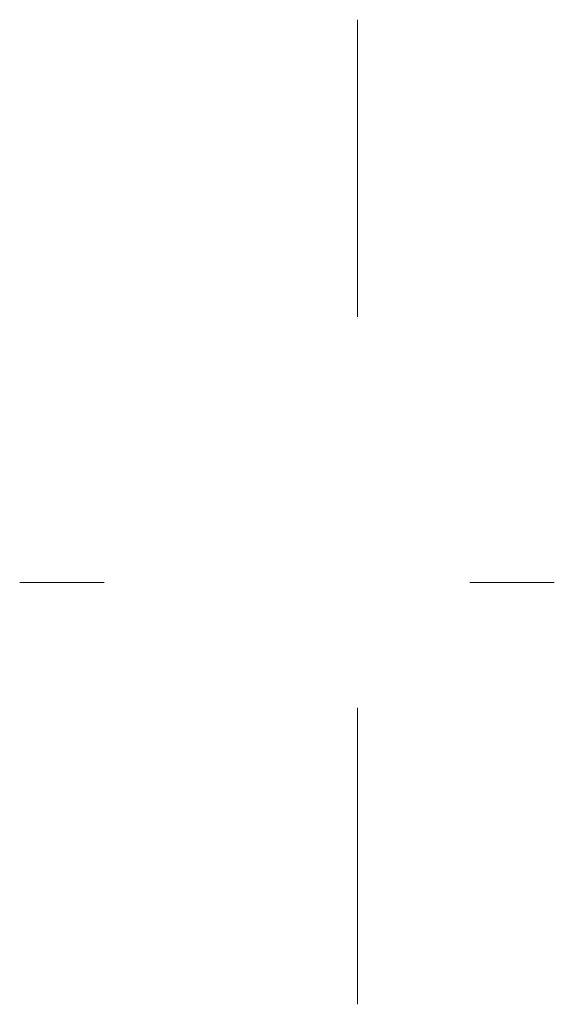
# Model space of a CAD drawing. Units: millimetres. Extents: x 248.5 to 267.5, y 286.2 to 321.2.
import ezdxf

# ---------------------------------------------------------------- set-up
doc = ezdxf.new("R2010")
doc.units = ezdxf.units.MM
doc.layers.add('M-CONS', color=8, linetype='Continuous', lineweight=13)

msp = doc.modelspace()

# ---------------------------------------------------------------- linework, layer by layer
at = {"layer": 'M-CONS'}
for p, q in [((260.455, 310.676, 64.753), (260.455, 321.239, 49.891)), ((248.455, 301.239, 54.82), (251.455, 301.239, 54.82)), ((251.455, 301.239, 54.82), (248.455, 301.239, 46.175)), ((267.455, 301.239, 54.82), (264.455, 301.239, 54.82)), ((264.455, 301.239, 54.82), (267.455, 301.239, 46.175)), ((260.455, 296.779, 64.753), (260.455, 286.239, 49.891))]:
    msp.add_line(p, q, dxfattribs=at)

doc.saveas('drawing.dxf')
